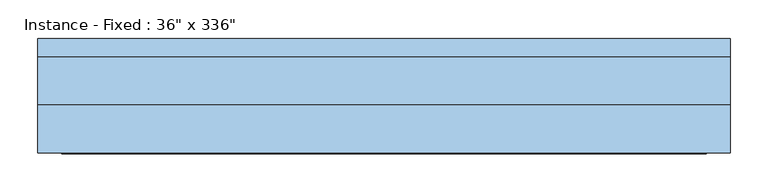
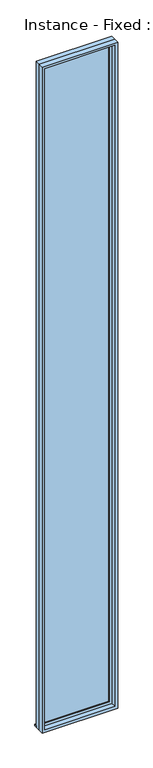
"""IFC4 building model written with IfcOpenShell, lengths in millimetres: window geometry."""

from ifc_helpers import new_model, si_unit, frame, origin, place, context, project, spatial, polyline, outline, extrude, source, transform, mapped, element, save


def window_9b859ad1(model_context):
    return source(origin(), model_context, "Body", "SweptSolid", [
        extrude(outline(polyline([(-495.3, 88.9), (419.1, 88.9), (419.1, 63.5), (-495.3, 63.5), (-495.3, 88.9)])), frame((0.0, 0.0, 914.4), z_axis=(0.0, 0.0, 1.0), x_axis=(1.0, 0.0, 0.0)), (0.0, 0.0, 1.0), 19.05),
        extrude(outline(polyline([(355.6, 15.875), (-431.8, 15.875), (-431.8, 28.575), (355.6, 28.575), (355.6, 15.875)])), frame((0.0, 0.0, 977.9), z_axis=(0.0, 0.0, 1.0), x_axis=(1.0, 0.0, 0.0)), (0.0, 0.0, 1.0), 8407.4),
        extrude(outline(polyline([(9429.75, -476.25), (933.45, -476.25), (933.45, 400.05), (9429.75, 400.05), (9429.75, -476.25)]), holes=[polyline([(9385.3, -431.8), (9385.3, 355.6), (977.9, 355.6), (977.9, -431.8), (9385.3, -431.8)])]), frame((0.0, 0.0, 0.0), z_axis=(0.0, 1.0, 0.0), x_axis=(0.0, 0.0, 1.0)), (0.0, 0.0, 1.0), 44.45),
        extrude(outline(polyline([(9448.8, -495.3), (914.4, -495.3), (914.4, 419.1), (9448.8, 419.1), (9448.8, -495.3)]), holes=[polyline([(9417.05, -463.55), (9417.05, 387.35), (946.15, 387.35), (946.15, -463.55), (9417.05, -463.55)])]), frame((0.0, -63.5, 0.0), z_axis=(0.0, 1.0, 0.0), x_axis=(0.0, 0.0, 1.0)), (0.0, 0.0, 1.0), 63.5),
        extrude(outline(polyline([(9448.8, 419.1), (9448.8, -495.3), (914.4, -495.3), (914.4, 419.1), (9448.8, 419.1)]), holes=[polyline([(9429.75, 400.05), (933.45, 400.05), (933.45, -476.25), (9429.75, -476.25), (9429.75, 400.05)])]), frame((0.0, 0.0, 0.0), z_axis=(0.0, 1.0, 0.0), x_axis=(0.0, 0.0, 1.0)), (0.0, 0.0, 1.0), 63.5),
    ])


if __name__ == "__main__":
    model = new_model("IFC4")
    model_context = context("Model", 3, world=origin())
    ifc_project = project(units=[si_unit("LENGTHUNIT", "METRE", prefix="MILLI")], contexts=[model_context])
    site = spatial("IfcSite", under=ifc_project)
    building = spatial("IfcBuilding", under=site)
    placement = place(None, origin())
    window_shape = window_9b859ad1(model_context)
    element("IfcWindow", 1, ObjectType="Instance - Fixed : 36\" x 336\"", at=placement, inside=building, context=model_context, shape_type="MappedRepresentation", body=[
        mapped(window_shape, transform((0.0, 0.0, 0.0), x_axis=(1.0, 0.0, 0.0), y_axis=(0.0, 1.0, 0.0), z_axis=(0.0, 0.0, 1.0))),
    ])
    save(model, "model.ifc")

# Revit data of these elements
# Type "Instance - Fixed : 36\" x 336\""
#   Type Mark = "10"
#   Construction Type Id = "GSP4R"
#   Assembly Code = "B2020100"
#   Analytic Construction = "1/8 in Pilkington single glazing"
#   Visual Light Transmittance = 0.9
#   Thermal Resistance (R) = 0.8466 (h·ft²·°F)/BTU
#   Solar Heat Gain Coefficient = 0.86
#   Heat Transfer Coefficient (U) = 1.1812 BTU/(h·ft²·°F)
#   Height [instance default] = 4' - 0"
#   Default Sill Height = 3' - 0"
#   Width [instance default] = 2' - 0"
#   Window Inset = 0' - 0 3/4"
#   Define Thermal Properties by = 1
#   Glass Pane Material = Glass
#   Sash Material = Sash
#   Wall Closure = (empty or 0)
# Element 1 (IfcWindow, "Instance - Fixed : 36\" x 336\"")
#   Height = 28' - 0"
#   Width = 3' - 0"
#   Materials on its faces: "Sash", "Glass"
# Materials
#   "Glass": class "Glass", colour RGB 0 128 192, transparency 0.75, Description = "Soda Lime Glass", Cost = 0
#   "Sash": class "Wood", colour RGB 224 178 126, transparency 0
